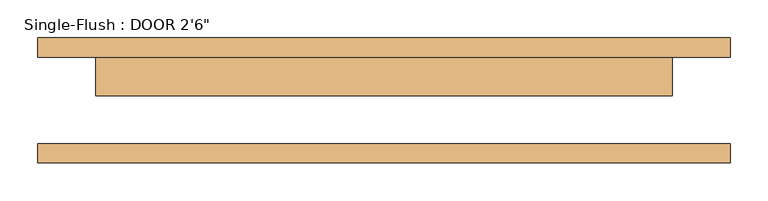
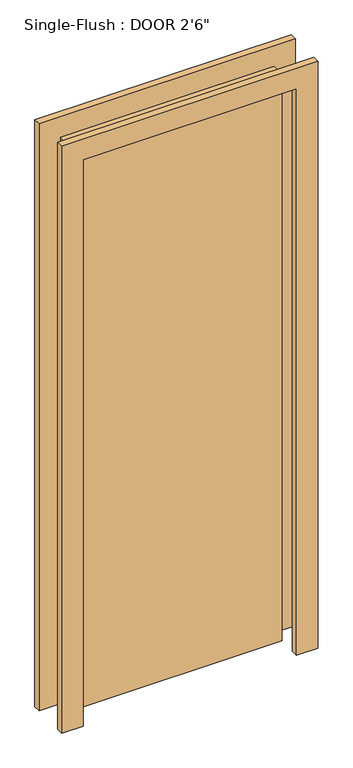
"""IFC4 building model written with IfcOpenShell, lengths in millimetres: door geometry."""

from ifc_helpers import new_model, si_unit, frame, origin, origin_with_axes, place, context, project, spatial, polyline, outline, extrude, source, transform, mapped, element, save


def door_214872d5(model_context):
    return source(origin(), model_context, "Body", "SweptSolid", [
        extrude(outline(polyline([(2209.8, -457.2), (0.0, -457.2), (0.0, -381.0), (2133.6, -381.0), (2133.6, 381.0), (0.0, 381.0), (0.0, 457.2), (2209.8, 457.2), (2209.8, -457.2)])), frame((0.0, 57.15, 0.0), z_axis=(0.0, 1.0, 0.0), x_axis=(0.0, 0.0, 1.0)), (0.0, 0.0, 1.0), 25.4),
        extrude(outline(polyline([(2209.8, 457.2), (2209.8, -457.2), (0.0, -457.2), (0.0, -381.0), (2133.6, -381.0), (2133.6, 381.0), (0.0, 381.0), (0.0, 457.2), (2209.8, 457.2)])), frame((0.0, -82.55, 0.0), z_axis=(0.0, 1.0, 0.0), x_axis=(0.0, 0.0, 1.0)), (0.0, 0.0, 1.0), 25.4),
        extrude(outline(polyline([(381.0, 6.35), (-381.0, 6.35), (-381.0, 57.15), (381.0, 57.15), (381.0, 6.35)])), origin_with_axes(), (0.0, 0.0, 1.0), 2133.6),
    ])


if __name__ == "__main__":
    model = new_model("IFC4")
    model_context = context("Model", 3, world=origin())
    ifc_project = project(units=[si_unit("LENGTHUNIT", "METRE", prefix="MILLI")], contexts=[model_context])
    site = spatial("IfcSite", under=ifc_project)
    building = spatial("IfcBuilding", under=site)
    placement = place(None, origin())
    door_shape = door_214872d5(model_context)
    element("IfcDoor", 1, ObjectType="Single-Flush : DOOR 2'6\"", at=placement, inside=building, context=model_context, shape_type="MappedRepresentation", body=[
        mapped(door_shape, transform((0.0, 0.0, 0.0), x_axis=(1.0, 0.0, 0.0), y_axis=(0.0, 1.0, 0.0), z_axis=(0.0, 0.0, 1.0))),
    ])
    save(model, "model.ifc")

# Revit data of these elements
# Type "Single-Flush : DOOR 2'6\""
#   Type Mark = "9"
#   Construction Type Id = "MDOOR"
#   Assembly Code = "C1020"
#   Analytic Construction = "Metal"
#   Thickness = 0' - 2"
#   Heat Transfer Coefficient (U) = 0.651978 BTU/(h·ft²·°F)
#   Height = 7' - 0"
#   Trim Projection Ext = 0' - 1"
#   Trim Projection Int = 0' - 1"
#   Trim Width = 0' - 3"
#   Width = 2' - 6"
#   Define Thermal Properties by = 1
#   Door Material = Door - Panel
#   Frame Material = Door - Frame
#   Visual Light Transmittance = 0
#   Solar Heat Gain Coefficient = 0
#   Function = (empty or 0)
#   Wall Closure = (empty or 0)
# Element 1 (IfcDoor, "Single-Flush : DOOR 2'6\"")
#   Materials on its faces: "Door - Frame", "Door - Panel"
# Materials
#   "Door - Panel": class "Wood", colour RGB 210 159 95, transparency 0, Cost = 0
#   "Door - Frame": colour RGB 118 70 51, transparency 0, Cost = 0
